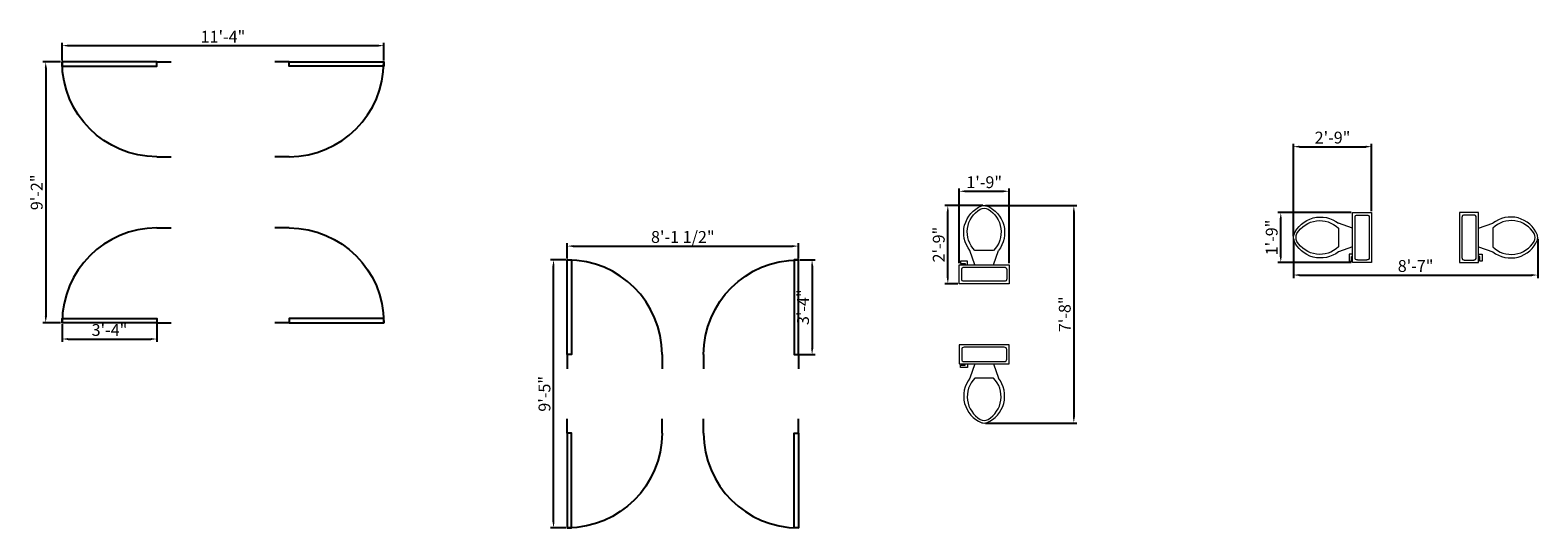
# Model space of a CAD drawing. Units: inches. Extents: x 351 to 1945, y 4338 to 4989.
# Tile 4 of 4: x 1308 to 1945, y 4779 to 4989. Entities that reach past the tile are written whole.
import ezdxf

# ---------------------------------------------------------------- set-up
doc = ezdxf.new("R2010")
doc.units = ezdxf.units.IN
for name, color, linetype, lineweight in [('A-ANNO-DIMS', 55, 'Continuous', 18), ('A-FLOR-FIXT', 9, 'Continuous', 18), ('DOOR', 52, 'Continuous', 25)]:
    doc.layers.add(name, color=color, linetype=linetype, lineweight=lineweight)
doc.styles.get("Standard").update_dxf_attribs({"font": 'arial.ttf'})
doc.dimstyles.new('ISO-25', dxfattribs={"dimtxt": 5, "dimasz": 2.5, "dimexe": 1.25, "dimexo": 0.625, "dimtad": 1, "dimdec": 0, "dimlunit": 4, "dimtxsty": 'Standard', "dimcen": 2.5, "dimadec": 0, "dimazin": 0, "dimtfac": 1, "dimtdec": 0, "dimtmove": 0, "dimatfit": 3, "dimfxl": 1, "dimarcsym": 0})

# ---------------------------------------------------------------- blocks, each defined once
blk = doc.blocks.new('*U2')
for p, q in [((0, 0), (0, -6)), ((40, 0), (40, -6))]:
    blk.add_line(p, q)
blk.add_lwpolyline([(0, 0), (0, 40), (1.75, 40), (1.75, 0)], close=True)
blk.add_arc((0, 0), 40, 0, 90)
blk = doc.blocks.new('*U4')
for p, q in [((9.5, -6), (9.5, -2)), ((-10, -8.5), (-8, -8.5)), ((-10, -9.5), (-10, -8.5)), ((-7, -9.5), (-10, -9.5)), ((-8, -8.5), (-8, -8)), ((-7, -8), (-7, -9.5)), ((-4, -8), (-6, -14)), ((4, -8), (6, -14)), ((4, -14), (-4, -14))]:
    blk.add_line(p, q)
blk.add_lwpolyline([(10.5, -8), (10.5, 0), (-10.5, 0), (-10.5, -8)], close=True)
for points in [[(-9.5, -2), (-9.5, -6)], [(8.5, -1), (-8.5, -1)], [(-8.5, -7), (8.5, -7)]]:
    blk.add_lwpolyline(points)
for centre, radius, start, end in [((-8.62, -1.88), 0.884, 81.8699, 188.1301), ((-8.62, -6.12), 0.884, 171.8699, 278.1301), ((8.62, -1.88), 0.884, 351.8699, 98.1301), ((8.62, -6.12), 0.884, 261.8699, 8.1301), ((3.52, -21.58), 12.17, 141.46911, 247.97143), ((4.2, -21.82), 11.33, 136.36773, 238.94682), ((-3.52, -21.58), 12.17, 292.02843, 38.53071), ((-4.2, -21.82), 11.33, 301.05301, 43.63209), ((0, -27.88), 4, 245.73182, 294.26817), ((0, -29), 4, 254.86053, 285.13947)]:
    blk.add_arc(centre, radius, start, end)
blk = doc.blocks.new('*D40')
at = {"layer": 'A-ANNO-DIMS', "color": 0, "lineweight": -2, "transparency": 16777216}
for p, q in [((1321.91, 4976.06), (1321.91, 4983.59)), ((1457.72, 4976.06), (1457.72, 4983.59)), ((1324.41, 4982.34), (1455.22, 4982.34))]:
    blk.add_line(p, q, dxfattribs=at)
at = {"layer": 'A-ANNO-DIMS', "color": 0, "lineweight": 100, "transparency": 16777216}
for points in [[(1324.41, 4982.75), (1324.41, 4981.92), (1321.91, 4982.34)], [(1455.22, 4982.75), (1455.22, 4981.92), (1457.72, 4982.34)]]:
    blk.add_solid(points, dxfattribs=at)
at = {"layer": 'Defpoints', "color": 0, "lineweight": 100, "transparency": 16777216}
for p in [(1457.72, 4982.34), (1321.91, 4975.44), (1457.72, 4975.44)]:
    blk.add_point(p, dxfattribs=at)
at = {"layer": 'A-ANNO-DIMS', "color": 0, "transparency": 16777216, "insert": (1389.81, 4985.47), "char_height": 5, "attachment_point": 5}
blk.add_mtext('11\'-4"', dxfattribs=at)
blk = doc.blocks.new('*D41')
at = {"layer": 'A-ANNO-DIMS', "color": 0, "lineweight": -2, "transparency": 16777216}
for p, q in [((1321.29, 4975.44), (1313.76, 4975.44)), ((1315.01, 4972.94), (1315.01, 4867.88)), ((1321.29, 4865.38), (1313.76, 4865.38))]:
    blk.add_line(p, q, dxfattribs=at)
at = {"layer": 'A-ANNO-DIMS', "color": 0, "lineweight": 100, "transparency": 16777216}
for points in [[(1314.6, 4972.94), (1315.43, 4972.94), (1315.01, 4975.44)], [(1314.6, 4867.88), (1315.43, 4867.88), (1315.01, 4865.38)]]:
    blk.add_solid(points, dxfattribs=at)
at = {"layer": 'Defpoints', "color": 0, "lineweight": 100, "transparency": 16777216}
for p in [(1321.91, 4975.44), (1315.01, 4865.38), (1321.91, 4865.38)]:
    blk.add_point(p, dxfattribs=at)
at = {"layer": 'A-ANNO-DIMS', "color": 0, "transparency": 16777216, "insert": (1311.84, 4920.41), "char_height": 5, "attachment_point": 5, "rotation": 90}
blk.add_mtext('9\'-2"', dxfattribs=at)
blk = doc.blocks.new('*D42')
at = {"layer": 'A-ANNO-DIMS', "color": 0, "lineweight": -2, "transparency": 16777216}
for p, q in [((1321.91, 4864.75), (1321.91, 4857.23)), ((1361.91, 4866.5), (1361.91, 4857.23)), ((1324.41, 4858.48), (1359.41, 4858.48))]:
    blk.add_line(p, q, dxfattribs=at)
at = {"layer": 'A-ANNO-DIMS', "color": 0, "lineweight": 100, "transparency": 16777216}
for points in [[(1324.41, 4858.9), (1324.41, 4858.06), (1321.91, 4858.48)], [(1359.41, 4858.9), (1359.41, 4858.06), (1361.91, 4858.48)]]:
    blk.add_solid(points, dxfattribs=at)
at = {"layer": 'Defpoints', "color": 0, "lineweight": 100, "transparency": 16777216}
for p in [(1321.91, 4865.38), (1361.91, 4867.13), (1361.91, 4858.48)]:
    blk.add_point(p, dxfattribs=at)
at = {"layer": 'A-ANNO-DIMS', "color": 0, "transparency": 16777216, "insert": (1341.91, 4861.66), "char_height": 5, "attachment_point": 5}
blk.add_mtext('3\'-4"', dxfattribs=at)
blk = doc.blocks.new('*D43')
at = {"layer": 'A-ANNO-DIMS', "color": 0, "lineweight": -2, "transparency": 16777216}
for p, q in [((1535.17, 4892.54), (1535.17, 4898.96)), ((1537.67, 4897.71), (1630.22, 4897.71)), ((1632.72, 4892.54), (1632.72, 4898.96))]:
    blk.add_line(p, q, dxfattribs=at)
at = {"layer": 'A-ANNO-DIMS', "color": 0, "lineweight": 100, "transparency": 16777216}
for points in [[(1537.67, 4898.13), (1537.67, 4897.3), (1535.17, 4897.71)], [(1630.22, 4898.13), (1630.22, 4897.3), (1632.72, 4897.71)]]:
    blk.add_solid(points, dxfattribs=at)
at = {"layer": 'Defpoints', "color": 0, "lineweight": 100, "transparency": 16777216}
for p in [(1632.72, 4897.71), (1535.17, 4891.91), (1632.72, 4891.91)]:
    blk.add_point(p, dxfattribs=at)
at = {"layer": 'A-ANNO-DIMS', "color": 0, "transparency": 16777216, "insert": (1583.94, 4900.92), "char_height": 5, "attachment_point": 5}
blk.add_mtext('8\'-1 1/2"', dxfattribs=at)
blk = doc.blocks.new('*D44')
at = {"layer": 'A-ANNO-DIMS', "color": 0, "lineweight": -2, "transparency": 16777216}
for p, q in [((1534.54, 4891.91), (1528.12, 4891.91)), ((1529.37, 4781.27), (1529.37, 4889.41)), ((1534.54, 4778.77), (1528.12, 4778.77))]:
    blk.add_line(p, q, dxfattribs=at)
at = {"layer": 'A-ANNO-DIMS', "color": 0, "lineweight": 100, "transparency": 16777216}
for points in [[(1528.95, 4889.41), (1529.78, 4889.41), (1529.37, 4891.91)], [(1528.95, 4781.27), (1529.78, 4781.27), (1529.37, 4778.77)]]:
    blk.add_solid(points, dxfattribs=at)
at = {"layer": 'Defpoints', "color": 0, "lineweight": 100, "transparency": 16777216}
for p in [(1529.37, 4891.91), (1535.17, 4891.91), (1535.17, 4778.77)]:
    blk.add_point(p, dxfattribs=at)
at = {"layer": 'A-ANNO-DIMS', "color": 0, "transparency": 16777216, "insert": (1526.19, 4835.34), "char_height": 5, "attachment_point": 5, "rotation": 90}
blk.add_mtext('9\'-5"', dxfattribs=at)
blk = doc.blocks.new('*D45')
at = {"layer": 'A-ANNO-DIMS', "color": 0, "lineweight": -2, "transparency": 16777216}
for p, q in [((1633.35, 4891.91), (1639.77, 4891.91)), ((1638.52, 4889.41), (1638.52, 4854.41)), ((1631.6, 4851.91), (1639.77, 4851.91))]:
    blk.add_line(p, q, dxfattribs=at)
at = {"layer": 'A-ANNO-DIMS', "color": 0, "lineweight": 100, "transparency": 16777216}
for points in [[(1638.11, 4889.41), (1638.94, 4889.41), (1638.52, 4891.91)], [(1638.11, 4854.41), (1638.94, 4854.41), (1638.52, 4851.91)]]:
    blk.add_solid(points, dxfattribs=at)
at = {"layer": 'Defpoints', "color": 0, "lineweight": 100, "transparency": 16777216}
for p in [(1632.72, 4891.91), (1630.97, 4851.91), (1638.52, 4851.91)]:
    blk.add_point(p, dxfattribs=at)
at = {"layer": 'A-ANNO-DIMS', "color": 0, "transparency": 16777216, "insert": (1635.34, 4871.91), "char_height": 5, "attachment_point": 5, "rotation": 90}
blk.add_mtext('3\'-4"', dxfattribs=at)
blk = doc.blocks.new('*D46')
at = {"layer": 'A-ANNO-DIMS', "color": 0, "lineweight": -2, "transparency": 16777216}
for p, q in [((1700.66, 4890.47), (1700.66, 4922.1)), ((1703.16, 4920.85), (1719.16, 4920.85)), ((1721.66, 4890.47), (1721.66, 4922.1))]:
    blk.add_line(p, q, dxfattribs=at)
at = {"layer": 'A-ANNO-DIMS', "color": 0, "lineweight": 100, "transparency": 16777216}
for points in [[(1703.16, 4921.27), (1703.16, 4920.44), (1700.66, 4920.85)], [(1719.16, 4921.27), (1719.16, 4920.44), (1721.66, 4920.85)]]:
    blk.add_solid(points, dxfattribs=at)
at = {"layer": 'Defpoints', "color": 0, "lineweight": 100, "transparency": 16777216}
for p in [(1721.66, 4920.85), (1700.66, 4889.84), (1721.66, 4889.84)]:
    blk.add_point(p, dxfattribs=at)
at = {"layer": 'A-ANNO-DIMS', "color": 0, "transparency": 16777216, "insert": (1711.16, 4924.03), "char_height": 5, "attachment_point": 5}
blk.add_mtext('1\'-9"', dxfattribs=at)
blk = doc.blocks.new('*D47')
at = {"layer": 'A-ANNO-DIMS', "color": 0, "lineweight": -2, "transparency": 16777216}
for p, q in [((1711.78, 4914.84), (1750.26, 4914.84)), ((1749.01, 4912.34), (1749.01, 4825.5)), ((1711.78, 4823), (1750.26, 4823))]:
    blk.add_line(p, q, dxfattribs=at)
at = {"layer": 'A-ANNO-DIMS', "color": 0, "lineweight": 100, "transparency": 16777216}
for points in [[(1748.59, 4912.34), (1749.42, 4912.34), (1749.01, 4914.84)], [(1748.59, 4825.5), (1749.42, 4825.5), (1749.01, 4823)]]:
    blk.add_solid(points, dxfattribs=at)
at = {"layer": 'Defpoints', "color": 0, "lineweight": 100, "transparency": 16777216}
for p in [(1711.16, 4914.84), (1711.16, 4823), (1749.01, 4823)]:
    blk.add_point(p, dxfattribs=at)
at = {"layer": 'A-ANNO-DIMS', "color": 0, "transparency": 16777216, "insert": (1745.83, 4868.92), "char_height": 5, "attachment_point": 5, "rotation": 90}
blk.add_mtext('7\'-8"', dxfattribs=at)
blk = doc.blocks.new('*D48')
at = {"layer": 'A-ANNO-DIMS', "color": 0, "lineweight": -2, "transparency": 16777216}
for p, q in [((1710.53, 4914.84), (1694.56, 4914.84)), ((1695.81, 4884.34), (1695.81, 4912.34)), ((1700.03, 4881.84), (1694.56, 4881.84))]:
    blk.add_line(p, q, dxfattribs=at)
at = {"layer": 'A-ANNO-DIMS', "color": 0, "lineweight": 100, "transparency": 16777216}
for points in [[(1695.39, 4912.34), (1696.22, 4912.34), (1695.81, 4914.84)], [(1695.39, 4884.34), (1696.22, 4884.34), (1695.81, 4881.84)]]:
    blk.add_solid(points, dxfattribs=at)
at = {"layer": 'Defpoints', "color": 0, "lineweight": 100, "transparency": 16777216}
for p in [(1695.81, 4914.84), (1711.16, 4914.84), (1700.66, 4881.84)]:
    blk.add_point(p, dxfattribs=at)
at = {"layer": 'A-ANNO-DIMS', "color": 0, "transparency": 16777216, "insert": (1692.63, 4898.34), "char_height": 5, "attachment_point": 5, "rotation": 90}
blk.add_mtext('2\'-9"', dxfattribs=at)
blk = doc.blocks.new('*D49')
at = {"layer": 'A-ANNO-DIMS', "color": 0, "lineweight": -2, "transparency": 16777216}
for p, q in [((1841.71, 4900.72), (1841.71, 4884.24)), ((1944.84, 4900.72), (1944.84, 4884.24)), ((1844.21, 4885.49), (1942.34, 4885.49))]:
    blk.add_line(p, q, dxfattribs=at)
at = {"layer": 'A-ANNO-DIMS', "color": 0, "lineweight": 100, "transparency": 16777216}
for points in [[(1844.21, 4885.91), (1844.21, 4885.08), (1841.71, 4885.49)], [(1942.34, 4885.91), (1942.34, 4885.08), (1944.84, 4885.49)]]:
    blk.add_solid(points, dxfattribs=at)
at = {"layer": 'Defpoints', "color": 0, "lineweight": 100, "transparency": 16777216}
for p in [(1841.71, 4901.34), (1944.84, 4901.34), (1944.84, 4885.49)]:
    blk.add_point(p, dxfattribs=at)
at = {"layer": 'A-ANNO-DIMS', "color": 0, "transparency": 16777216, "insert": (1893.27, 4888.67), "char_height": 5, "attachment_point": 5}
blk.add_mtext('8\'-7"', dxfattribs=at)
blk = doc.blocks.new('*D50')
at = {"layer": 'A-ANNO-DIMS', "color": 0, "lineweight": -2, "transparency": 16777216}
for p, q in [((1866.08, 4911.84), (1835.11, 4911.84)), ((1836.36, 4893.34), (1836.36, 4909.34)), ((1866.08, 4890.84), (1835.11, 4890.84))]:
    blk.add_line(p, q, dxfattribs=at)
at = {"layer": 'A-ANNO-DIMS', "color": 0, "lineweight": 100, "transparency": 16777216}
for points in [[(1835.94, 4909.34), (1836.77, 4909.34), (1836.36, 4911.84)], [(1835.94, 4893.34), (1836.77, 4893.34), (1836.36, 4890.84)]]:
    blk.add_solid(points, dxfattribs=at)
at = {"layer": 'Defpoints', "color": 0, "lineweight": 100, "transparency": 16777216}
for p in [(1836.36, 4911.84), (1866.71, 4911.84), (1866.71, 4890.84)]:
    blk.add_point(p, dxfattribs=at)
at = {"layer": 'A-ANNO-DIMS', "color": 0, "transparency": 16777216, "insert": (1833.18, 4901.34), "char_height": 5, "attachment_point": 5, "rotation": 90}
blk.add_mtext('1\'-9"', dxfattribs=at)
blk = doc.blocks.new('*D51')
at = {"layer": 'A-ANNO-DIMS', "color": 0, "lineweight": -2, "transparency": 16777216}
for p, q in [((1841.71, 4901.97), (1841.71, 4940.94)), ((1844.21, 4939.69), (1872.21, 4939.69)), ((1874.71, 4912.47), (1874.71, 4940.94))]:
    blk.add_line(p, q, dxfattribs=at)
at = {"layer": 'A-ANNO-DIMS', "color": 0, "lineweight": 100, "transparency": 16777216}
for points in [[(1844.21, 4940.11), (1844.21, 4939.28), (1841.71, 4939.69)], [(1872.21, 4940.11), (1872.21, 4939.28), (1874.71, 4939.69)]]:
    blk.add_solid(points, dxfattribs=at)
at = {"layer": 'Defpoints', "color": 0, "lineweight": 100, "transparency": 16777216}
for p in [(1874.71, 4939.69), (1874.71, 4911.84), (1841.71, 4901.34)]:
    blk.add_point(p, dxfattribs=at)
at = {"layer": 'A-ANNO-DIMS', "color": 0, "transparency": 16777216, "insert": (1858.21, 4942.87), "char_height": 5, "attachment_point": 5}
blk.add_mtext('2\'-9"', dxfattribs=at)

msp = doc.modelspace()

# ---------------------------------------------------------------- block references
at = {"layer": 'A-FLOR-FIXT', "xscale": -1}
for p, rotation in [((1711.16, 4881.84), 180), ((1874.71, 4901.34), 270)]:
    msp.add_blockref('*U4', p, dxfattribs=dict(at, rotation=rotation))
at = {"layer": 'A-FLOR-FIXT', "rotation": 90.00000000000003}
msp.add_blockref('*U4', (1911.84, 4901.34), dxfattribs=at)
at = {"layer": 'A-FLOR-FIXT'}
msp.add_blockref('*U4', (1711.16, 4856), dxfattribs=at)
at = {"layer": 'DOOR', "xscale": -1}
for p, rotation in [((1361.91, 4975.44), 90), ((1417.72, 4865.38), 270), ((1535.17, 4818.77), 180)]:
    msp.add_blockref('*U2', p, dxfattribs=dict(at, rotation=rotation))
at = {"layer": 'DOOR'}
for p, rotation in [((1417.72, 4975.44), 270), ((1361.91, 4865.38), 90), ((1632.72, 4818.77), 180)]:
    msp.add_blockref('*U2', p, dxfattribs=dict(at, rotation=rotation))
msp.add_blockref('*U2', (1535.17, 4851.91), dxfattribs=at)
at = {"layer": 'DOOR', "xscale": -1}
msp.add_blockref('*U2', (1632.72, 4851.91), dxfattribs=at)

# ---------------------------------------------------------------- dimensions: what is measured, and where the dimension line sits
at = {"layer": 'A-ANNO-DIMS'}
for base, p1, p2, picture, middle in [((1457.72, 4982.34), (1321.91, 4975.44), (1457.72, 4975.44), '*D40', (1389.81, 4985.47)), ((1874.71, 4939.69), (1841.71, 4901.34), (1874.71, 4911.84), '*D51', (1858.21, 4942.87)), ((1721.66, 4920.85), (1700.66, 4889.84), (1721.66, 4889.84), '*D46', (1711.16, 4924.03)), ((1632.7223, 4897.7147), (1535.1677, 4891.9147), (1632.7223, 4891.9147), '*D43', (1583.945, 4900.925)), ((1944.84, 4885.49), (1841.71, 4901.34), (1944.84, 4901.34), '*D49', (1893.27, 4888.67)), ((1361.91, 4858.48), (1321.91, 4865.38), (1361.91, 4867.13), '*D42', (1341.91, 4861.66))]:
    dim = msp.add_linear_dim(base=base, p1=p1, p2=p2, dimstyle='ISO-25', override={"dimdec": 1, "dimlfac": 1, "dimrnd": 0, "dimzin": 1, "dimdsep": 46, "dimlunit": 4, "dimfrac": 2}, dxfattribs=at)
    dim.commit()
    dim.dimension.update_dxf_attribs({"geometry": picture, "text_midpoint": middle})
for base, p1, p2, picture, middle in [((1315.01, 4865.38), (1321.91, 4975.44), (1321.91, 4865.38), '*D41', (1311.84, 4920.41)), ((1695.81, 4914.84), (1700.66, 4881.84), (1711.16, 4914.84), '*D48', (1692.63, 4898.34)), ((1749.01, 4823), (1711.16, 4914.84), (1711.16, 4823), '*D47', (1745.83, 4868.92)), ((1836.36, 4911.84), (1866.71, 4890.84), (1866.71, 4911.84), '*D50', (1833.18, 4901.34)), ((1529.37, 4891.91), (1535.17, 4778.77), (1535.17, 4891.91), '*D44', (1526.19, 4835.34)), ((1638.52, 4851.91), (1632.72, 4891.91), (1630.97, 4851.91), '*D45', (1635.34, 4871.91))]:
    dim = msp.add_linear_dim(base=base, p1=p1, p2=p2, angle=90, dimstyle='ISO-25', override={"dimdec": 1, "dimlfac": 1, "dimrnd": 0, "dimzin": 1, "dimdsep": 46, "dimlunit": 4, "dimfrac": 2}, dxfattribs=at)
    dim.commit()
    dim.dimension.update_dxf_attribs({"geometry": picture, "text_midpoint": middle})

doc.saveas('drawing.dxf')
